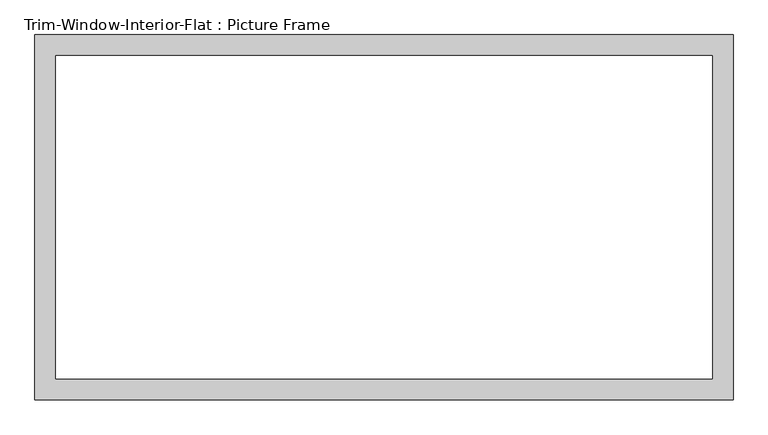
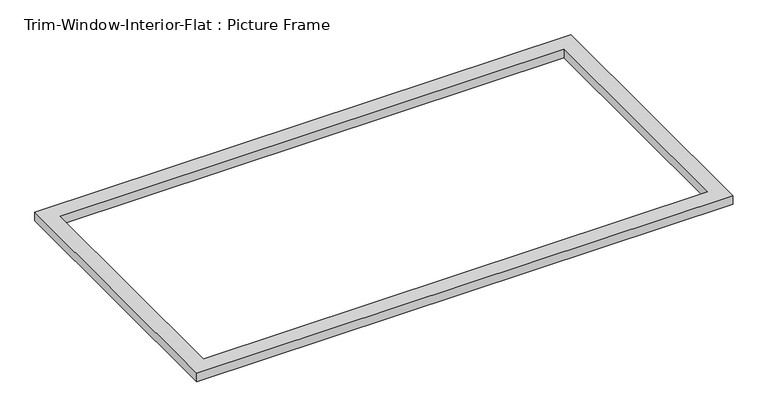
"""IFC4 building model written with IfcOpenShell, lengths in millimetres: proxy geometry, Trim-Window-Interior-Flat : Picture Frame."""

from ifc_helpers import new_model, si_unit, origin, origin_with_axes, place, context, project, spatial, polyline, outline, extrude, source, transform, mapped, element, save


def trim_window_interior_flat_picture_frame_0edfbaa2(model_context):
    return source(origin(), model_context, "Body", "SweptSolid", [
        extrude(outline(polyline([(958.85, 44.45), (958.85, -958.85), (-958.85, -958.85), (-958.85, 44.45), (958.85, 44.45)]), holes=[polyline([(901.7, -12.7), (-901.7, -12.7), (-901.7, -901.7), (901.7, -901.7), (901.7, -12.7)])]), origin_with_axes(), (0.0, 0.0, 1.0), 31.75),
    ])


if __name__ == "__main__":
    model = new_model("IFC4")
    model_context = context("Model", 3, world=origin())
    ifc_project = project(units=[si_unit("LENGTHUNIT", "METRE", prefix="MILLI")], contexts=[model_context])
    site = spatial("IfcSite", under=ifc_project)
    building = spatial("IfcBuilding", under=site)
    placement = place(None, origin())
    trim_window_interior_flat_picture_frame_shape = trim_window_interior_flat_picture_frame_0edfbaa2(model_context)
    element("IfcBuildingElementProxy", 1, Name="Trim-Window-Interior-Flat : Picture Frame", ObjectType="Trim-Window-Interior-Flat : Picture Frame", at=placement, inside=building, context=model_context, shape_type="MappedRepresentation", body=[
        mapped(trim_window_interior_flat_picture_frame_shape, transform((0.0, 0.0, 0.0), x_axis=(1.0, 0.0, 0.0), y_axis=(0.0, 1.0, 0.0), z_axis=(0.0, 0.0, 1.0))),
    ])
    save(model, "model.ifc")

# Revit data of these elements
# Type "Trim-Window-Interior-Flat : Picture Frame"
#   Trim Thickness_Picture Frame = 0.104167 ft
#   Trim Width = 0.1875 ft
#   Trim Thickness_with Sill = 0.0625 ft
#   Sill Thickness = 0.104167 ft
#   Opening Width [instance default] = 2 ft
#   Opening Height [instance default] = 3 ft
#   Default Elevation = 4 ft
#   Sill = no
#   Picture Frame = yes
#   Trim Material [instance default] = none
# Element 1 (IfcBuildingElementProxy, "Trim-Window-Interior-Flat : Picture Frame")
#   Opening Width = 6 ft
#   Trim Material = Wood - Stained
#   Materials on its faces: "Wood - Stained"
# Materials
#   "Wood - Stained": class "Wood", colour RGB 224 178 126, transparency 0, Cost = 0
